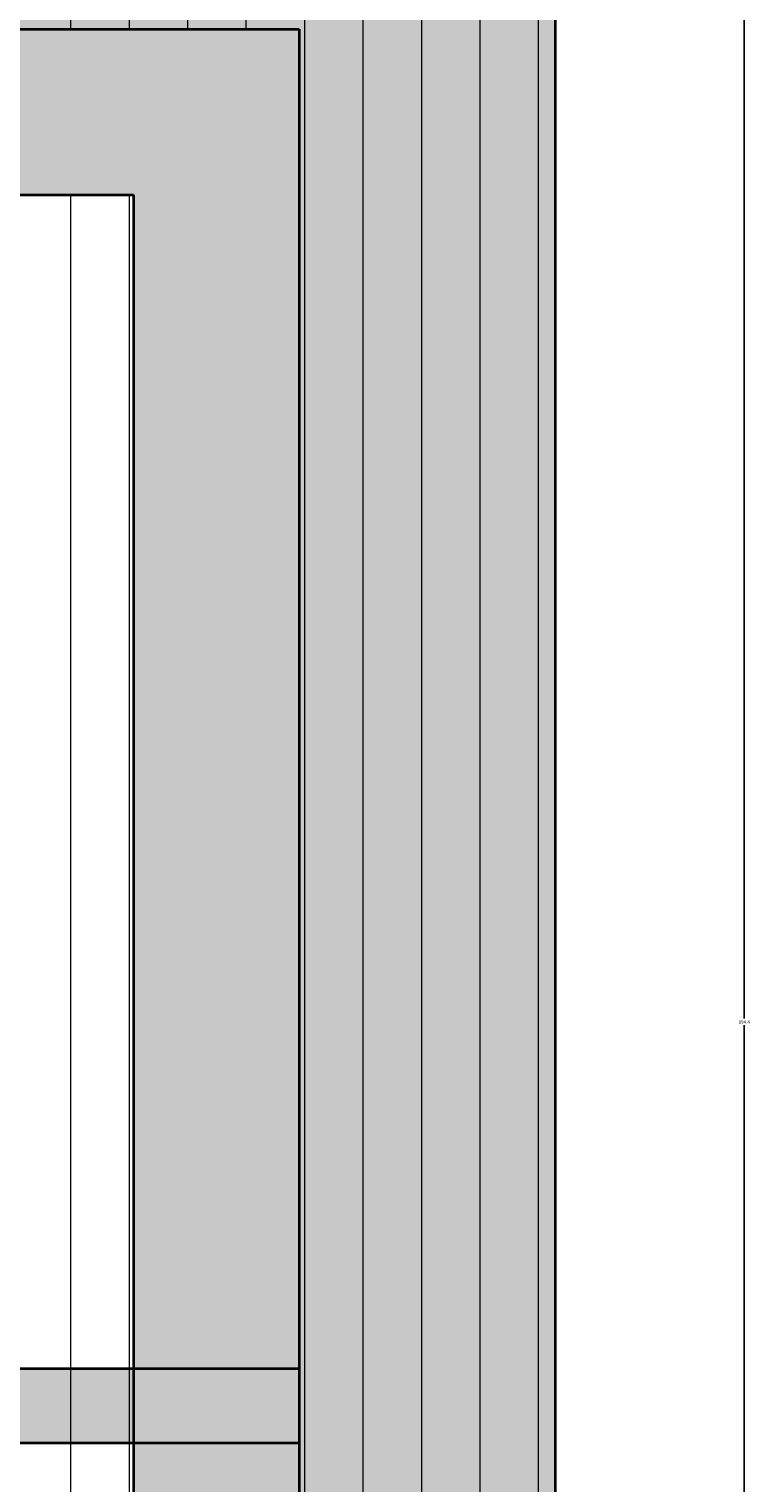
# Model space of a CAD drawing. Units: millimetres. Extents: x 446512 to 447461, y 70395 to 70610.
# Tile 26 of 39: x 447016 to 447055, y 70477 to 70556. Entities that reach past the tile are written whole.
import ezdxf

# ---------------------------------------------------------------- set-up
doc = ezdxf.new("R2010")
doc.units = ezdxf.units.MM
for name, color, linetype, lineweight in [('A-ANNO-DIMS', 2, 'Continuous', 18), ('A-FURN', 7, 'Continuous', 35), ('A-FURN-PATT', 38, 'Continuous', 13)]:
    doc.layers.add(name, color=color, linetype=linetype, lineweight=lineweight)
doc.styles.get("Standard").update_dxf_attribs({"font": 'arial.ttf'})
doc.dimstyles.get("Standard").update_dxf_attribs({"dimtxt": 0.18, "dimasz": 0.18, "dimexe": 0.18, "dimexo": 0.0625, "dimgap": 0.09, "dimtad": 0, "dimtih": 1, "dimtoh": 1, "dimdec": 4, "dimzin": 0, "dimdsep": 46, "dimtxsty": 'Standard', "dimcen": 0.09, "dimadec": 0, "dimazin": 0, "dimtfac": 1, "dimtdec": 4, "dimtofl": 0, "dimtmove": 0, "dimatfit": 3, "dimfxl": 1, "dimtolj": 1, "dimtzin": 0, "dimarcsym": 0})

# ---------------------------------------------------------------- blocks, each defined once
blk = doc.blocks.new('*D52')
at = {"layer": 'A-ANNO-DIMS', "color": 0, "lineweight": -2, "transparency": 16777216}
for p, q in [((447044.159, 70599.715), (447054.526, 70599.715)), ((447054.346, 70599.535), (447054.346, 70502.696)), ((447054.346, 70405.495), (447054.346, 70502.333)), ((447044.159, 70405.315), (447054.526, 70405.315))]:
    blk.add_line(p, q, dxfattribs=at)
at = {"layer": 'A-ANNO-DIMS', "color": 0, "transparency": 16777216}
for points in [[(447054.316, 70599.535), (447054.376, 70599.535), (447054.346, 70599.715)], [(447054.316, 70405.495), (447054.376, 70405.495), (447054.346, 70405.315)]]:
    blk.add_solid(points, dxfattribs=at)
at = {"layer": 'Defpoints', "color": 0, "transparency": 16777216}
for p in [(447044.096, 70599.715), (447054.346, 70599.715), (447044.096, 70405.315)]:
    blk.add_point(p, dxfattribs=at)
at = {"layer": 'A-ANNO-DIMS', "color": 0, "transparency": 16777216, "insert": (447054.346, 70502.515), "char_height": 0.18, "attachment_point": 5}
blk.add_mtext('\\A1;194.4', dxfattribs=at)

msp = doc.modelspace()

# ---------------------------------------------------------------- hatches: boundary and pattern name
at = {"layer": 'A-FURN-PATT'}
h = msp.add_hatch(dxfattribs=at)
h.set_pattern_fill('ANSI31', color=256, angle=45)
h.paths.add_polyline_path([(447044.0961, 70599.7147), (446983.5069, 70599.7147), (446983.5069, 70556.4508), (447030.1693, 70556.4508), (447030.1693, 70442.4508), (446983.5069, 70442.4508), (446983.5069, 70405.3145), (447044.0961, 70405.3145)])
h.paths.add_polyline_path([(447021.1693, 70547.4508), (446983.5069, 70547.4508), (446983.5069, 70451.4508), (447021.1693, 70451.4508)], flags=17)
h = msp.add_hatch(color=256, dxfattribs=at)
h.dxf.hatch_style = 1
h.paths.add_polyline_path([(447021.1693, 70483.6935), (446983.5069, 70483.6935), (446983.5069, 70479.6272), (447021.1693, 70479.6272)], flags=17)
h.paths.add_polyline_path([(447030.1693, 70483.6935), (447021.1693, 70483.6935), (447021.1693, 70479.6272), (447030.1693, 70479.6272)], flags=17)
h.paths.add_polyline_path([(447044.0961, 70599.7147), (446983.5069, 70599.7147), (446983.5069, 70556.4508), (447030.1693, 70556.4508), (447030.1693, 70442.4508), (446983.5069, 70442.4508), (446983.5069, 70405.3145), (447044.0961, 70405.3145)])
h = msp.add_hatch(color=256, dxfattribs=at)
h.dxf.hatch_style = 1
h.paths.add_polyline_path([(446983.5069, 70556.4508), (446964.1693, 70556.4508), (446964.1693, 70442.4508), (446983.5069, 70442.4508), (446983.5069, 70451.4508), (446973.1693, 70451.4508), (446973.1693, 70547.4508), (446983.5069, 70547.4508)])
h.paths.add_polyline_path([(447030.1693, 70556.4508), (446983.5069, 70556.4508), (446983.5069, 70547.4508), (447021.1693, 70547.4508), (447021.1693, 70451.4508), (446983.5069, 70451.4508), (446983.5069, 70442.4508), (447030.1693, 70442.4508)])
h = msp.add_hatch(color=256, dxfattribs=at)
h.dxf.hatch_style = 1
h.paths.add_polyline_path([(447030.1693, 70483.6935), (447021.1693, 70483.6935), (447021.1693, 70479.6272), (447030.1693, 70479.6272)])

# ---------------------------------------------------------------- linework, layer by layer
at = {"layer": 'A-FURN'}
msp.add_line((447044.0961, 70405.3145), (447044.0961, 70599.7147), dxfattribs=at)
for points in [[(447030.1693, 70556.4508), (447030.1693, 70442.4508), (446964.1693, 70442.4508), (446964.1693, 70556.4508)], [(447021.1693, 70547.4508), (447021.1693, 70451.4508), (446973.1693, 70451.4508), (446973.1693, 70547.4508)], [(446964.1693, 70483.6935), (447030.1693, 70483.6935), (447030.1693, 70479.6272), (446964.1693, 70479.6272)]]:
    msp.add_lwpolyline(points, close=True, dxfattribs=at)

# ---------------------------------------------------------------- dimensions: what is measured, and where the dimension line sits
at = {"layer": 'A-ANNO-DIMS'}
dim = msp.add_linear_dim(base=(447054.3461, 70599.7147), p1=(447044.0961, 70405.3145), p2=(447044.0961, 70599.7147), angle=90, dimstyle='Standard', override={"dimdec": 1, "dimlfac": 1, "dimrnd": 0, "dimzin": 0, "dimdsep": 46, "dimlunit": 2}, dxfattribs=at)
dim.commit()
dim.dimension.update_dxf_attribs({"geometry": '*D52', "text_midpoint": (447054.3461, 70502.5146)})

doc.saveas('drawing.dxf')
